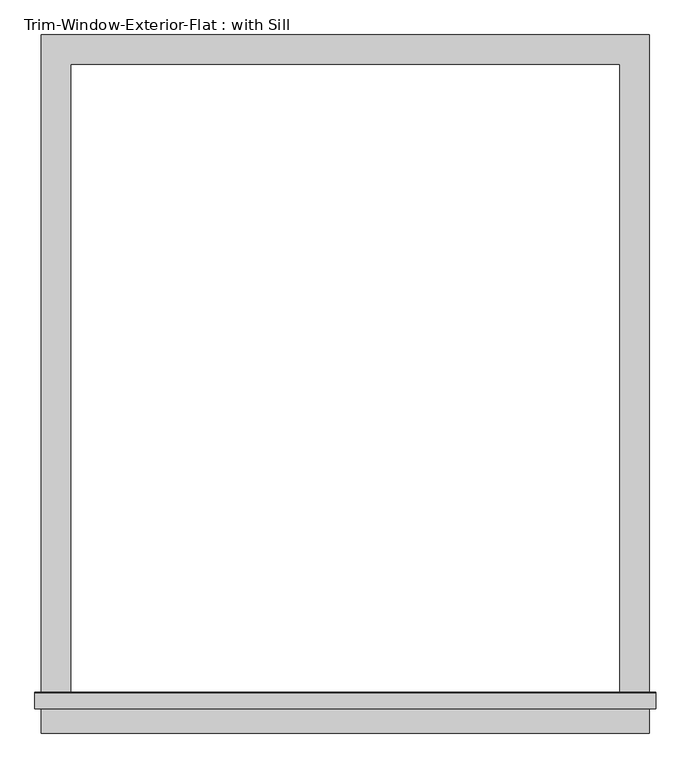
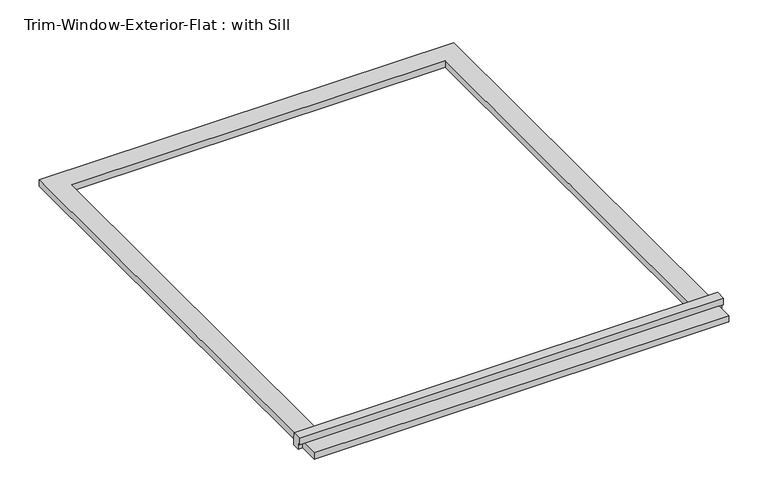
"""IFC4 building model written with IfcOpenShell, lengths in millimetres: proxy geometry, Trim-Window-Exterior-Flat : with Sill."""

from ifc_helpers import new_model, si_unit, frame, origin, origin_with_axes, place, context, project, spatial, polyline, outline, extrude, source, transform, mapped, element, save


def trim_window_exterior_flat_with_sill_245f2bb1(model_context):
    return source(origin(), model_context, "Body", "SweptSolid", [
        extrude(outline(polyline([(590.55, -1241.3823709), (590.55, -1298.5323709), (-590.55, -1298.5323709), (-590.55, -1241.3823709), (590.55, -1241.3823709)])), origin_with_axes(), (0.0, 0.0, 1.0), 19.05),
        extrude(outline(polyline([(-1250.95, 38.1), (-1221.6580645, 38.1), (-1219.2, 19.05), (-1219.2, 0.0), (-1241.3823709, 0.0), (-1241.3823709, 19.05), (-1250.95, 19.05), (-1250.95, 38.1)])), frame((-603.25, 0.0, 0.0), z_axis=(1.0, 0.0, 0.0), x_axis=(0.0, 1.0, 0.0)), (0.0, 0.0, 1.0), 1206.5),
        extrude(outline(polyline([(-590.55, 57.15), (590.55, 57.15), (590.55, -1219.2), (533.4, -1219.2), (533.4, 0.0), (-533.4, 0.0), (-533.4, -1219.2), (-590.55, -1219.2), (-590.55, 57.15)])), origin_with_axes(), (0.0, 0.0, 1.0), 19.05),
    ])


if __name__ == "__main__":
    model = new_model("IFC4")
    model_context = context("Model", 3, world=origin())
    ifc_project = project(units=[si_unit("LENGTHUNIT", "METRE", prefix="MILLI")], contexts=[model_context])
    site = spatial("IfcSite", under=ifc_project)
    building = spatial("IfcBuilding", under=site)
    placement = place(None, origin())
    trim_window_exterior_flat_with_sill_shape = trim_window_exterior_flat_with_sill_245f2bb1(model_context)
    element("IfcBuildingElementProxy", 1, Name="Trim-Window-Exterior-Flat : with Sill", ObjectType="Trim-Window-Exterior-Flat : with Sill", at=placement, inside=building, context=model_context, shape_type="MappedRepresentation", body=[
        mapped(trim_window_exterior_flat_with_sill_shape, transform((0.0, 0.0, 0.0), x_axis=(1.0, 0.0, 0.0), y_axis=(0.0, 1.0, 0.0), z_axis=(0.0, 0.0, 1.0))),
    ])
    save(model, "model.ifc")

# Revit data of these elements
# Type "Trim-Window-Exterior-Flat : with Sill"
#   Trim Width = 0' - 2 1/4"
#   Trim Thickness_Picture Frame = 0' - 1 1/4"
#   Trim Thickness_with Sill = 0' - 0 3/4"
#   Sill Thickness = 0' - 1 1/4"
#   Opening Width [instance default] = 2' - 0"
#   Opening Height [instance default] = 3' - 0"
#   Default Elevation = 4' - 0"
#   Sill = yes
#   Picture Frame = no
#   Trim Material [instance default] = none
# Element 1 (IfcBuildingElementProxy, "Trim-Window-Exterior-Flat : with Sill")
#   Opening Width = 3' - 6"
#   Opening Height = 4' - 0"
#   Trim Material = Clad - White
#   Materials on its faces: "Clad - White"
# Materials
#   "Clad - White": class "Wood", colour RGB 242 242 238, transparency 0, Cost = 0
